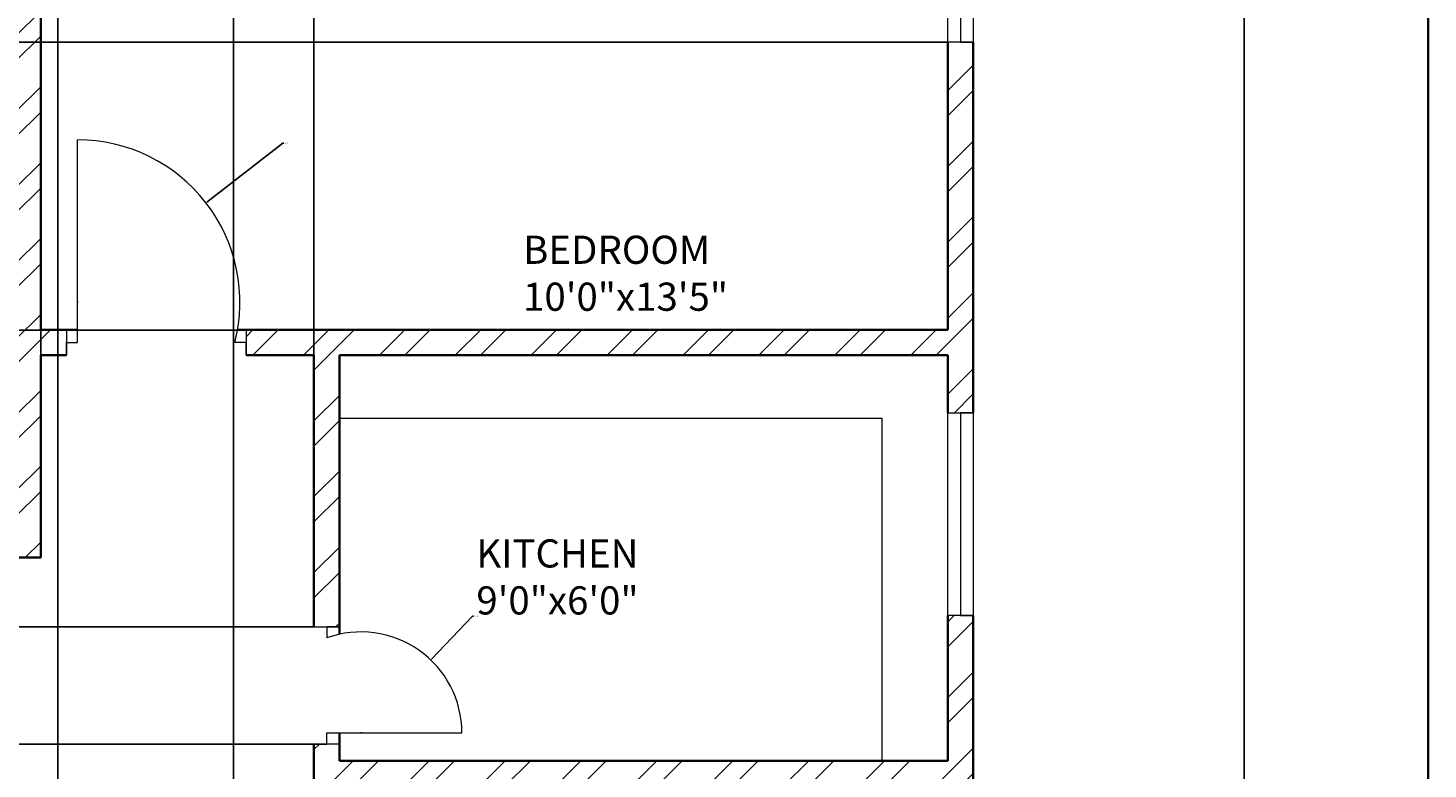
# Model space of a CAD drawing. Units: inches. Extents: x 2008 to 2657, y 1077 to 2165.
# Tile 15 of 16: x 2409 to 2657, y 1805 to 1937. Entities that reach past the tile are written whole.
import ezdxf

# ---------------------------------------------------------------- set-up
doc = ezdxf.new("R2010")
doc.units = ezdxf.units.IN
for name, color, linetype, lineweight in [('A-ANNO-DIMS', 2, 'Continuous', 18), ('A-ANNO-TTLB', 7, 'Continuous', 35), ('A-AREA-IDEN', 4, 'Continuous', 18), ('A-DOOR', 11, 'Continuous', 18), ('A-FLOR-CASE', 9, 'Continuous', 18), ('A-GLAZ', 191, 'Continuous', 18), ('A-WALL', 7, 'Continuous', 35)]:
    doc.layers.add(name, color=color, linetype=linetype, lineweight=lineweight)
doc.layers.add('A-WALL-PATT', color=30, linetype='Continuous', lineweight=13, true_color=0xf8991e)
doc.styles.get("Standard").update_dxf_attribs({"font": 'arial.ttf'})
doc.dimstyles.get("Standard").update_dxf_attribs({"dimtxt": 0.18, "dimasz": 0.18, "dimexe": 0.18, "dimexo": 0.0625, "dimgap": 0.09, "dimtad": 0, "dimtih": 1, "dimtoh": 1, "dimdec": 4, "dimzin": 0, "dimdsep": 46, "dimtxsty": 'Standard', "dimcen": 0.09, "dimadec": 0, "dimazin": 0, "dimtfac": 1, "dimtdec": 4, "dimtofl": 0, "dimtmove": 0, "dimatfit": 3, "dimfxl": 1, "dimtolj": 1, "dimtzin": 0, "dimarcsym": 0})

# ---------------------------------------------------------------- blocks, each defined once
blk = doc.blocks.new('WIN-60IN-B')
for p, q in [((0, 4.5), (0, 0)), ((0, 4.5), (60, 4.5)), ((60, 2.25), (60, 4.5)), ((60, 4.5), (60, 0)), ((0, 0), (0, 2.25)), ((0, 2.25), (60, 2.25)), ((60, 0), (0, 0))]:
    blk.add_line(p, q)
blk = doc.blocks.new('WIN-36IN-A')
for p, q in [((0, 36), (4.5, 36)), ((0, 0), (0, 36)), ((4.5, 36), (2.25, 36)), ((2.25, 36), (2.25, 0)), ((4.5, 36), (4.5, 0)), ((4.5, 0), (0, 0)), ((2.25, 0), (4.5, 0))]:
    blk.add_line(p, q)
blk = doc.blocks.new('*D32')
at = {"layer": 'A-ANNO-DIMS', "color": 0, "lineweight": -2, "transparency": 16777216}
for p, q in [((2576.82, 2094.67), (2624.99, 2094.67)), ((2624.81, 2094.49), (2624.81, 1641.86)), ((2624.81, 1188.85), (2624.81, 1641.49)), ((2576.82, 1188.67), (2624.99, 1188.67))]:
    blk.add_line(p, q, dxfattribs=at)
at = {"layer": 'A-ANNO-DIMS', "color": 0, "transparency": 16777216}
for points in [[(2624.78, 2094.49), (2624.84, 2094.49), (2624.81, 2094.67)], [(2624.78, 1188.85), (2624.84, 1188.85), (2624.81, 1188.67)]]:
    blk.add_solid(points, dxfattribs=at)
at = {"layer": 'Defpoints', "color": 0, "transparency": 16777216}
for p in [(2576.76, 2094.67), (2624.81, 2094.67), (2576.76, 1188.67)]:
    blk.add_point(p, dxfattribs=at)
at = {"layer": 'A-ANNO-DIMS', "color": 0, "transparency": 16777216, "insert": (2624.81, 1641.67), "char_height": 0.18, "attachment_point": 5}
blk.add_mtext('\\A1;906', dxfattribs=at)
blk = doc.blocks.new('*D56')
at = {"layer": 'A-ANNO-DIMS', "color": 0, "lineweight": -2, "transparency": 16777216}
for p, q in [((2411.26, 1842.83), (2411.26, 2142.9)), ((2411.44, 2142.72), (2435.18, 2142.72)), ((2459.58, 2142.72), (2435.84, 2142.72)), ((2459.76, 1830.56), (2459.76, 2142.9))]:
    blk.add_line(p, q, dxfattribs=at)
at = {"layer": 'A-ANNO-DIMS', "color": 0, "transparency": 16777216}
for points in [[(2411.44, 2142.75), (2411.44, 2142.69), (2411.26, 2142.72)], [(2459.58, 2142.75), (2459.58, 2142.69), (2459.76, 2142.72)]]:
    blk.add_solid(points, dxfattribs=at)
at = {"layer": 'Defpoints', "color": 0, "transparency": 16777216}
for p in [(2459.76, 2142.72), (2411.26, 1842.77), (2459.76, 1830.5)]:
    blk.add_point(p, dxfattribs=at)
at = {"layer": 'A-ANNO-DIMS', "color": 0, "transparency": 16777216, "insert": (2435.51, 2142.72), "char_height": 0.18, "attachment_point": 5}
blk.add_mtext('\\A1;48.5', dxfattribs=at)
blk = doc.blocks.new('*D57')
at = {"layer": 'A-ANNO-DIMS', "color": 0, "lineweight": -2, "transparency": 16777216}
for p, q in [((2414.28, 1754.24), (2414.28, 2142.9)), ((2414.46, 2142.72), (2429.47, 2142.72)), ((2445.27, 2142.72), (2430.26, 2142.72)), ((2445.45, 1751.99), (2445.45, 2142.9))]:
    blk.add_line(p, q, dxfattribs=at)
at = {"layer": 'A-ANNO-DIMS', "color": 0, "transparency": 16777216}
for points in [[(2414.46, 2142.75), (2414.46, 2142.69), (2414.28, 2142.72)], [(2445.27, 2142.75), (2445.27, 2142.69), (2445.45, 2142.72)]]:
    blk.add_solid(points, dxfattribs=at)
at = {"layer": 'Defpoints', "color": 0, "transparency": 16777216}
for p in [(2445.45, 2142.72), (2414.28, 1754.17), (2445.45, 1751.92)]:
    blk.add_point(p, dxfattribs=at)
at = {"layer": 'A-ANNO-DIMS', "color": 0, "transparency": 16777216, "insert": (2429.87, 2142.72), "char_height": 0.18, "attachment_point": 5}
blk.add_mtext('\\A1;31.17', dxfattribs=at)
blk = doc.blocks.new('*D58')
at = {"layer": 'A-ANNO-DIMS', "color": 0, "lineweight": -2, "transparency": 16777216}
for p, q in [((2459.7, 1830.5), (2028.03, 1830.5)), ((2028.21, 1830.32), (2028.21, 1820.26)), ((2028.21, 1809.84), (2028.21, 1819.9)), ((2459.7, 1809.66), (2028.03, 1809.66))]:
    blk.add_line(p, q, dxfattribs=at)
at = {"layer": 'A-ANNO-DIMS', "color": 0, "transparency": 16777216}
for points in [[(2028.18, 1830.32), (2028.24, 1830.32), (2028.21, 1830.5)], [(2028.18, 1809.84), (2028.24, 1809.84), (2028.21, 1809.66)]]:
    blk.add_solid(points, dxfattribs=at)
at = {"layer": 'Defpoints', "color": 0, "transparency": 16777216}
for p in [(2028.21, 1830.5), (2459.76, 1830.5), (2459.76, 1809.66)]:
    blk.add_point(p, dxfattribs=at)
at = {"layer": 'A-ANNO-DIMS', "color": 0, "transparency": 16777216, "insert": (2028.21, 1820.08), "char_height": 0.18, "attachment_point": 5}
blk.add_mtext('\\A1;20.835', dxfattribs=at)
blk = doc.blocks.new('*D67')
at = {"layer": 'A-ANNO-DIMS', "color": 0, "lineweight": -2, "transparency": 16777216}
for p, q in [((2572.2, 1934.29), (2028.03, 1934.29)), ((2028.21, 1934.11), (2028.21, 1908.91)), ((2028.21, 1883.35), (2028.21, 1908.55)), ((2572.2, 1883.17), (2028.03, 1883.17))]:
    blk.add_line(p, q, dxfattribs=at)
at = {"layer": 'A-ANNO-DIMS', "color": 0, "transparency": 16777216}
for points in [[(2028.18, 1934.11), (2028.24, 1934.11), (2028.21, 1934.29)], [(2028.18, 1883.35), (2028.24, 1883.35), (2028.21, 1883.17)]]:
    blk.add_solid(points, dxfattribs=at)
at = {"layer": 'Defpoints', "color": 0, "transparency": 16777216}
for p in [(2028.21, 1934.29), (2572.26, 1934.29), (2572.26, 1883.17)]:
    blk.add_point(p, dxfattribs=at)
at = {"layer": 'A-ANNO-DIMS', "color": 0, "transparency": 16777216, "insert": (2028.21, 1908.73), "char_height": 0.18, "attachment_point": 5}
blk.add_mtext('\\A1;51.11', dxfattribs=at)
blk = doc.blocks.new('*D72')
at = {"layer": 'A-ANNO-DIMS', "color": 0, "lineweight": -2, "transparency": 16777216}
for p, q in [((2454.25, 1916.34), (2440.73, 1905.87)), ((2454.43, 1916.34), (2454.25, 1916.34)), ((2417.73, 1888.13), (2417.91, 1888.13)), ((2417.82, 1888.04), (2417.82, 1888.22))]:
    blk.add_line(p, q, dxfattribs=at)
at = {"layer": 'A-ANNO-DIMS', "color": 0, "transparency": 16777216}
blk.add_solid([(2440.71, 1905.89), (2440.75, 1905.85), (2440.59, 1905.76)], dxfattribs=at)
at = {"layer": 'Defpoints', "color": 0, "transparency": 16777216}
for p in [(2440.59, 1905.76), (2417.82, 1888.13)]:
    blk.add_point(p, dxfattribs=at)
at = {"layer": 'A-ANNO-DIMS', "color": 0, "transparency": 16777216, "insert": (2454.84, 1916.34), "char_height": 0.18, "attachment_point": 5}
blk.add_mtext('\\A1;R28.8', dxfattribs=at)
blk = doc.blocks.new('*D88')
at = {"layer": 'A-ANNO-DIMS', "color": 0, "lineweight": -2, "transparency": 16777216}
for p, q in [((2487.89, 1832.39), (2480.59, 1824.74)), ((2488.07, 1832.39), (2487.89, 1832.39)), ((2468.02, 1811.66), (2468.2, 1811.66)), ((2468.11, 1811.57), (2468.11, 1811.75))]:
    blk.add_line(p, q, dxfattribs=at)
at = {"layer": 'A-ANNO-DIMS', "color": 0, "transparency": 16777216}
blk.add_solid([(2480.57, 1824.77), (2480.62, 1824.72), (2480.47, 1824.61)], dxfattribs=at)
at = {"layer": 'Defpoints', "color": 0, "transparency": 16777216}
for p in [(2480.47, 1824.61), (2468.11, 1811.66)]:
    blk.add_point(p, dxfattribs=at)
at = {"layer": 'A-ANNO-DIMS', "color": 0, "transparency": 16777216, "insert": (2488.62, 1832.39), "char_height": 0.18, "attachment_point": 5}
blk.add_mtext('\\A1;R17.905', dxfattribs=at)

msp = doc.modelspace()

# ---------------------------------------------------------------- hatches: boundary and pattern name
at = {"layer": 'A-WALL-PATT'}
h = msp.add_hatch(dxfattribs=at)
h.set_pattern_fill('ANSI32', color=256)
h.paths.add_polyline_path([(2109.2619, 2094.6743), (2104.7619, 2094.6743), (2104.7619, 2072.1743), (2104.7619, 2021.6151), (2109.2619, 2021.6151), (2109.2619, 2055.6743), (2126.1387, 2055.6743), (2126.1387, 2057.9243), (2126.1387, 2060.1743), (2109.2619, 2060.1743)])
h.paths.add_polyline_path([(2223.2494, 2057.9243), (2223.2494, 2060.1743), (2186.1387, 2060.1743), (2186.1387, 2055.6743), (2223.2494, 2055.6743)])
h.paths.add_polyline_path([(2250.7619, 2072.1743), (2250.7619, 2090.1743), (2250.7619, 2094.6743), (2246.2619, 2094.6743), (2246.2619, 2060.1743), (2242.7242, 2060.1743), (2242.7242, 2055.6743), (2246.2619, 2055.6743), (2246.2619, 1899.6743), (2242.7458, 1899.6743), (2242.7458, 1897.4243), (2242.7458, 1895.1743), (2246.2619, 1895.1743), (2246.2619, 1878.8745), (2248.5119, 1878.8745), (2250.7619, 1878.8745), (2250.7619, 1991.1743), (2250.7619, 2025.6743), (2257.6798, 2025.6743), (2257.6798, 2027.9243), (2257.6798, 2030.1743), (2250.7619, 2030.1743)])
h.paths.add_polyline_path([(2411.2619, 2031.6743), (2409.0119, 2031.6743), (2406.7619, 2031.6743), (2406.7619, 2030.1743), (2322.7619, 2030.1743), (2322.7619, 2053.3443), (2318.2619, 2053.3443), (2318.2619, 2030.1743), (2305.6798, 2030.1743), (2305.6798, 2025.6743), (2318.2619, 2025.6743), (2322.7619, 2025.6743), (2406.7619, 2025.6743), (2406.7619, 1995.6743), (2406.7619, 1847.2677), (2250.7619, 1847.2677), (2250.7619, 1850.9902), (2248.5119, 1850.9902), (2246.2619, 1850.9902), (2246.2619, 1847.1743), (2246.2619, 1842.7677), (2303.0015, 1842.7677), (2303.0015, 1667.2413), (2298.4208, 1667.2413), (2298.4208, 1662.7413), (2303.0015, 1662.7413), (2303.0015, 1649.8758), (2307.5015, 1649.8758), (2307.5015, 1842.7677), (2406.7619, 1842.7677), (2411.2619, 1842.7677), (2411.2619, 1878.6743), (2415.8196, 1878.6743), (2415.8196, 1880.9243), (2415.8196, 1883.1743), (2411.2619, 1883.1743)])
h.paths.add_polyline_path([(2411.2619, 2094.6743), (2406.7619, 2094.6743), (2318.2619, 2094.6743), (2318.2619, 2077.3443), (2322.7619, 2077.3443), (2322.7619, 2090.1743), (2406.7619, 2090.1743), (2406.7619, 2072.1743), (2406.7619, 2067.6743), (2406.7619, 2052.7524), (2411.2619, 2052.7524), (2411.2619, 2055.6743), (2414.9888, 2055.6743), (2414.9888, 2057.9243), (2414.9888, 2060.1743), (2411.2619, 2060.1743), (2411.2619, 2072.1743)])
h.paths.add_polyline_path([(2576.7619, 2072.1743), (2576.7619, 2094.6743), (2572.2619, 2094.6743), (2572.2619, 2060.1743), (2525.8113, 2060.1743), (2525.8113, 2055.6743), (2572.2619, 2055.6743), (2572.2619, 1994.289), (2576.7619, 1994.289)])
h.paths.add_polyline_path([(2465.8113, 2060.1743), (2436.2802, 2060.1743), (2436.2802, 2055.6743), (2465.8113, 2055.6743), (2465.8113, 2057.9243)])
h.paths.add_polyline_path([(2576.7619, 1934.289), (2574.5119, 1934.289), (2572.2619, 1934.289), (2572.2619, 1883.1743), (2447.7027, 1883.1743), (2447.7027, 1878.6743), (2459.7619, 1878.6743), (2459.7619, 1830.4982), (2464.2619, 1830.4982), (2464.2619, 1878.6743), (2572.2619, 1878.6743), (2572.2619, 1868.4883), (2576.7619, 1868.4883)])
h.paths.add_polyline_path([(2576.7619, 1832.4883), (2572.2619, 1832.4883), (2572.2619, 1806.6743), (2464.2619, 1806.6743), (2464.2619, 1809.6629), (2459.7619, 1809.6629), (2459.7619, 1802.1743), (2483.7619, 1802.1743), (2483.7619, 1778.1743), (2488.2619, 1778.1743), (2488.2619, 1802.1743), (2572.2619, 1802.1743), (2572.2619, 1793.6101), (2576.7619, 1793.6101)])
h.paths.add_polyline_path([(2576.7619, 1769.6101), (2572.2619, 1769.6101), (2572.2619, 1754.1743), (2488.2619, 1754.1743), (2488.2619, 1757.2675), (2486.0119, 1757.2675), (2483.7619, 1757.2675), (2483.7619, 1754.1743), (2447.4528, 1754.1743), (2447.4528, 1749.6743), (2483.7619, 1749.6743), (2572.2619, 1749.6743), (2572.2619, 1715.1837), (2576.7619, 1715.1837)])
h.paths.add_polyline_path([(2576.7619, 1655.1837), (2572.2619, 1655.1837), (2572.2619, 1617.6743), (2411.2619, 1617.6743), (2411.2619, 1749.6743), (2414.2827, 1749.6743), (2414.2827, 1754.1743), (2406.7619, 1754.1743), (2406.7619, 1749.6743), (2406.7619, 1617.6743), (2307.5015, 1617.6743), (2307.5015, 1621.0007), (2305.2515, 1621.0007), (2303.0015, 1621.0007), (2303.0015, 1609.6944), (2307.5015, 1609.6944), (2307.5015, 1613.1743), (2406.7619, 1613.1743), (2406.7619, 1476.6743), (2415.532, 1476.6743), (2415.532, 1478.9243), (2415.532, 1481.1743), (2411.2619, 1481.1743), (2411.2619, 1613.1743), (2572.2619, 1613.1743), (2572.2619, 1584.6086), (2576.7619, 1584.6086)])
h.paths.add_polyline_path([(2576.7619, 1524.6086), (2572.2619, 1524.6086), (2572.2619, 1481.1743), (2483.7619, 1481.1743), (2447.5119, 1481.1743), (2447.5119, 1476.6743), (2483.7619, 1476.6743), (2483.7619, 1473.5051), (2488.2619, 1473.5051), (2488.2619, 1476.6743), (2572.2619, 1476.6743), (2572.2619, 1469.5488), (2576.7619, 1469.5488)])
h.paths.add_polyline_path([(2576.7619, 1445.5488), (2572.2619, 1445.5488), (2572.2619, 1428.6743), (2488.2619, 1428.6743), (2488.2619, 1455.6743), (2486.0119, 1455.6743), (2483.7619, 1455.6743), (2483.7619, 1428.6743), (2459.7619, 1428.6743), (2459.7619, 1422.1519), (2464.2619, 1422.1519), (2464.2619, 1424.1743), (2572.2619, 1424.1743), (2572.2619, 1407.5685), (2576.7619, 1407.5685)])
h.paths.add_polyline_path([(2576.7619, 1371.5685), (2572.2619, 1371.5685), (2572.2619, 1352.1743), (2464.2619, 1352.1743), (2464.2619, 1403.1384), (2462.0119, 1403.1384), (2459.7619, 1403.1384), (2459.7619, 1352.1743), (2446.3194, 1352.1743), (2446.3194, 1347.6743), (2572.2619, 1347.6743), (2572.2619, 1321.0291), (2576.7619, 1321.0291)])
h.paths.add_polyline_path([(2462.703, 1227.6743), (2436.0298, 1227.6743), (2436.0298, 1225.4243), (2436.0298, 1223.1743), (2462.703, 1223.1743), (2462.703, 1225.4243)])
h.paths.add_polyline_path([(2576.7619, 1261.0291), (2574.5119, 1261.0291), (2572.2619, 1261.0291), (2572.2619, 1227.6743), (2522.703, 1227.6743), (2522.703, 1223.1743), (2572.2619, 1223.1743), (2572.2619, 1188.6743), (2576.7619, 1188.6743), (2576.7619, 1193.1743), (2576.7619, 1223.1743)])
h.paths.add_polyline_path([(2414.2823, 1227.6743), (2411.2619, 1227.6743), (2411.2619, 1267.1779), (2409.0119, 1267.1779), (2406.7619, 1267.1779), (2406.7619, 1227.6743), (2322.7619, 1227.6743), (2322.7619, 1244.3623), (2318.2619, 1244.3623), (2318.2619, 1223.1743), (2406.7619, 1223.1743), (2406.7619, 1193.1743), (2406.7619, 1188.6743), (2411.2619, 1188.6743), (2411.2619, 1193.1743), (2411.2619, 1223.1743), (2414.2823, 1223.1743)])
h.paths.add_polyline_path([(2411.2619, 1347.6743), (2414.702, 1347.6743), (2414.702, 1349.9243), (2414.702, 1352.1743), (2411.2619, 1352.1743), (2411.2619, 1416.7413), (2307.5015, 1416.7413), (2307.5015, 1579.8489), (2305.2515, 1579.8489), (2303.0015, 1579.8489), (2303.0015, 1566.7413), (2299.2719, 1566.7413), (2299.2719, 1562.2413), (2303.0015, 1562.2413), (2303.0015, 1416.7413), (2246.2619, 1416.7413), (2246.2619, 1409.8616), (2250.7619, 1409.8616), (2250.7619, 1412.2413), (2406.7619, 1412.2413), (2406.7619, 1292.1743), (2304.9703, 1292.1743), (2304.9703, 1287.6743), (2318.2619, 1287.6743), (2318.2619, 1268.3623), (2322.7619, 1268.3623), (2322.7619, 1287.6743), (2406.7619, 1287.6743), (2406.7619, 1285.4748), (2411.2619, 1285.4748)])
h.paths.add_polyline_path([(2109.2619, 1262.7482), (2104.7619, 1262.7482), (2104.7619, 1223.1743), (2104.7619, 1193.1743), (2104.7619, 1188.6743), (2109.2619, 1188.6743), (2109.2619, 1223.1743), (2126.7928, 1223.1743), (2126.7928, 1225.4243), (2126.7928, 1227.6743), (2109.2619, 1227.6743)])
h.paths.add_polyline_path([(2222.3268, 1227.6743), (2186.7928, 1227.6743), (2186.7928, 1223.1743), (2222.3268, 1223.1743)])
h.paths.add_polyline_path([(2250.7619, 1287.6743), (2256.9703, 1287.6743), (2256.9703, 1289.9243), (2256.9703, 1292.1743), (2250.7619, 1292.1743), (2250.7619, 1382.2078), (2248.5119, 1382.2078), (2246.2619, 1382.2078), (2246.2619, 1347.6743), (2246.2619, 1227.6743), (2242.6068, 1227.6743), (2242.6068, 1223.1743), (2246.2619, 1223.1743), (2246.2619, 1188.6743), (2250.7619, 1188.6743), (2250.7619, 1193.1743), (2250.7619, 1227.6743)])
h.paths.add_polyline_path([(2133.2619, 1349.9243), (2133.2619, 1352.1743), (2109.2619, 1352.1743), (2109.2619, 1375.2826), (2104.7619, 1375.2826), (2104.7619, 1322.7482), (2109.2619, 1322.7482), (2109.2619, 1347.6743), (2133.2619, 1347.6743)])
h.paths.add_polyline_path([(2210.2105, 1352.1743), (2161.7619, 1352.1743), (2161.7619, 1412.2413), (2185.7619, 1412.2413), (2185.7619, 1420.1851), (2183.5119, 1420.1851), (2181.2619, 1420.1851), (2181.2619, 1416.7413), (2109.2619, 1416.7413), (2109.2619, 1452.4006), (2104.7619, 1452.4006), (2104.7619, 1399.2826), (2109.2619, 1399.2826), (2109.2619, 1412.2413), (2157.2619, 1412.2413), (2157.2619, 1352.1743), (2154.3383, 1352.1743), (2154.3383, 1347.6743), (2210.2105, 1347.6743)])
h.paths.add_polyline_path([(2185.7619, 1514.2413), (2161.7619, 1514.2413), (2161.7619, 1518.1307), (2159.5119, 1518.1307), (2157.2619, 1518.1307), (2157.2619, 1514.2413), (2109.2619, 1514.2413), (2109.2619, 1528.997), (2107.0119, 1528.997), (2104.7619, 1528.997), (2104.7619, 1488.4006), (2109.2619, 1488.4006), (2109.2619, 1509.7413), (2181.2619, 1509.7413), (2181.2619, 1441.2042), (2185.7619, 1441.2042)])
h.paths.add_polyline_path([(2270.4025, 1566.7413), (2109.2619, 1566.7413), (2080.7619, 1566.7413), (2080.7619, 1586.5643), (2076.2619, 1586.5643), (2076.2619, 1562.2413), (2080.7619, 1562.2413), (2104.7619, 1562.2413), (2104.7619, 1552.997), (2109.2619, 1552.997), (2109.2619, 1562.2413), (2157.2619, 1562.2413), (2157.2619, 1538.2413), (2161.7619, 1538.2413), (2161.7619, 1562.2413), (2205.2619, 1562.2413), (2270.4025, 1562.2413)])
h.paths.add_polyline_path([(2131.6813, 1897.4243), (2131.6813, 1899.6743), (2109.2619, 1899.6743), (2109.2619, 1961.6151), (2104.7619, 1961.6151), (2104.7619, 1886.8042), (2109.2619, 1886.8042), (2109.2619, 1895.1743), (2131.6813, 1895.1743)])
h.paths.add_polyline_path([(2185.7619, 1847.1743), (2161.7619, 1847.1743), (2161.7619, 1895.1743), (2185.7619, 1895.1743), (2211.543, 1895.1743), (2211.543, 1897.4243), (2211.543, 1899.6743), (2154.0916, 1899.6743), (2154.0916, 1897.4243), (2154.0916, 1895.1743), (2157.2619, 1895.1743), (2157.2619, 1847.1743), (2109.2619, 1847.1743), (2109.2619, 1862.8042), (2104.7619, 1862.8042), (2104.7619, 1821.243), (2109.2619, 1821.243), (2109.2619, 1842.6743), (2181.2619, 1842.6743), (2181.2619, 1840.6763), (2185.7619, 1840.6763)])
h.paths.add_polyline_path([(2109.2619, 1785.243), (2104.7619, 1785.243), (2104.7619, 1715.4691), (2109.2619, 1715.4691), (2109.2619, 1730.8423), (2157.2619, 1730.8423), (2157.2619, 1727.6404), (2161.7619, 1727.6404), (2161.7619, 1730.8423), (2185.7619, 1730.8423), (2185.7619, 1822.1438), (2183.5119, 1822.1438), (2181.2619, 1822.1438), (2181.2619, 1735.3423), (2109.2619, 1735.3423)])
h.paths.add_polyline_path([(2109.2619, 1691.4691), (2104.7619, 1691.4691), (2104.7619, 1667.2413), (2076.2619, 1667.2413), (2076.2619, 1646.5643), (2080.7619, 1646.5643), (2080.7619, 1662.7413), (2109.2619, 1662.7413), (2271.4941, 1662.7413), (2271.4941, 1664.9913), (2271.4941, 1667.2413), (2181.2619, 1667.2413), (2161.7619, 1667.2413), (2161.7619, 1708.3752), (2159.5119, 1708.3752), (2157.2619, 1708.3752), (2157.2619, 1667.2413), (2109.2619, 1667.2413)])
h.paths.add_polyline_path([(2233.1467, 1747.4973), (2270.0737, 1747.4973), (2270.0737, 1766.1547), (2233.1467, 1766.1547)], flags=9)

# ---------------------------------------------------------------- linework, layer by layer
at = {"layer": 'A-ANNO-TTLB'}
msp.add_lwpolyline([(2008.4537, 2164.5615), (2657.4477, 2164.5615), (2657.4477, 1076.8888), (2008.4537, 1076.8888)], close=True, dxfattribs=at)
at = {"layer": 'A-DOOR'}
for p, q in [((2417.8196, 1880.9243), (2417.8196, 1916.9243)), ((2415.8196, 1883.1743), (2415.8196, 1878.6743)), ((2447.7027, 1883.1743), (2447.7027, 1878.6743)), ((2415.8196, 1878.6743), (2415.8196, 1880.9243)), ((2415.8196, 1880.9243), (2417.8196, 1880.9243)), ((2447.7027, 1880.9243), (2445.7027, 1880.9243)), ((2447.7027, 1878.6743), (2447.7027, 1880.9243)), ((2459.7619, 1830.4982), (2464.2619, 1830.4982)), ((2464.2619, 1830.4982), (2462.0119, 1830.4982)), ((2462.0119, 1830.4982), (2462.0119, 1828.4982)), ((2462.0119, 1809.6629), (2462.0119, 1811.6629)), ((2462.0119, 1811.6629), (2486.0119, 1811.6629)), ((2464.2619, 1809.6629), (2459.7619, 1809.6629)), ((2459.7619, 1809.6629), (2462.0119, 1809.6629))]:
    msp.add_line(p, q, dxfattribs=at)
for centre, radius, start, end in [((2417.8196, 1888.1262), 28.7981, 345.517596, 90), ((2468.1072, 1811.6629), 17.9047, 360, 109.902868)]:
    msp.add_arc(centre, radius, start, end, dxfattribs=at)
at = {"layer": 'A-FLOR-CASE'}
for p, q in [((2464.2619, 1867.5128), (2560.5188, 1867.5128)), ((2560.5188, 1867.5128), (2560.5188, 1806.6743))]:
    msp.add_line(p, q, dxfattribs=at)
at = {"layer": 'A-WALL'}
for p, q in [((2411.2619, 2031.6743), (2411.2619, 1883.1743)), ((2572.2619, 1934.289), (2572.2619, 1883.1743)), ((2576.7619, 1934.289), (2576.7619, 1868.4883)), ((2572.2619, 1895.1743), (2572.2619, 1883.1743)), ((2411.2619, 1883.1743), (2417.8196, 1883.1743)), ((2446.1888, 1883.1743), (2572.2619, 1883.1743)), ((2411.2619, 1878.6743), (2415.8196, 1878.6743)), ((2411.2619, 1878.6743), (2411.2619, 1842.7677)), ((2447.7027, 1878.6743), (2459.7619, 1878.6743)), ((2459.7619, 1878.6743), (2459.7619, 1830.4982)), ((2464.2619, 1878.6743), (2464.2619, 1829.1499)), ((2464.2619, 1878.6743), (2572.2619, 1878.6743)), ((2572.2619, 1878.6743), (2572.2619, 1868.4883)), ((2406.7619, 1842.7677), (2411.2619, 1842.7677)), ((2572.2619, 1832.4883), (2572.2619, 1806.6743)), ((2576.7619, 1832.4883), (2576.7619, 1793.6101)), ((2464.2619, 1811.6629), (2464.2619, 1806.6743)), ((2459.7619, 1809.6629), (2459.7619, 1802.1743)), ((2464.2619, 1806.6743), (2572.2619, 1806.6743))]:
    msp.add_line(p, q, dxfattribs=at)

# ---------------------------------------------------------------- block references
at = {"layer": 'A-GLAZ', "rotation": 270.0000000000001}
msp.add_blockref('WIN-60IN-B', (2572.2616, 1994.2888), dxfattribs=at)
at = {"layer": 'A-GLAZ'}
msp.add_blockref('WIN-36IN-A', (2572.262, 1832.488), dxfattribs=at)

# ---------------------------------------------------------------- texts
at = {"layer": 'A-AREA-IDEN', "char_height": 5, "attachment_point": 1}
for s, width, insert in [('BEDROOM\\P10\'0"x13\'5"', 135.75227, (2496.8689, 1899.9149)), ('KITCHEN\\P9\'0"x6\'0"', 165.62191, (2488.5766, 1846.0034))]:
    msp.add_mtext_dynamic_manual_height_columns(s, width=width, gutter_width=12.5, heights=[0], dxfattribs=dict(at, insert=insert))

# ---------------------------------------------------------------- dimensions: what is measured, and where the dimension line sits
at = {"layer": 'A-ANNO-DIMS'}
for base, p1, p2, override, picture, middle in [((2459.7619, 2142.7243), (2411.2619, 1842.7677), (2459.7619, 1830.4982), {"dimdec": 1, "dimlfac": 1, "dimrnd": 0, "dimzin": 0, "dimdsep": 46, "dimlunit": 2}, '*D56', (2435.5119, 2142.7243)), ((2445.4528, 2142.7243), (2414.2827, 1754.1743), (2445.4528, 1751.9243), {"dimdec": 2, "dimlfac": 1, "dimrnd": 0, "dimzin": 0, "dimdsep": 46, "dimlunit": 2}, '*D57', (2429.8677, 2142.7243))]:
    dim = msp.add_linear_dim(base=base, p1=p1, p2=p2, dimstyle='Standard', override=override, dxfattribs=at)
    dim.commit()
    dim.dimension.update_dxf_attribs({"geometry": picture, "text_midpoint": middle})
for base, p1, p2, override, picture, middle in [((2624.8119, 2094.6743), (2576.7619, 1188.6743), (2576.7619, 2094.6743), {"dimdec": 0, "dimlfac": 1, "dimrnd": 0, "dimzin": 0, "dimdsep": 46, "dimlunit": 2}, '*D32', (2624.8119, 1641.6743)), ((2028.2119, 1934.289), (2572.2619, 1883.1743), (2572.2619, 1934.289), {"dimdec": 2, "dimlfac": 1, "dimrnd": 0, "dimzin": 0, "dimdsep": 46, "dimlunit": 2}, '*D67', (2028.2119, 1908.7317)), ((2028.2119, 1830.4982), (2459.7619, 1809.6629), (2459.7619, 1830.4982), {"dimdec": 3, "dimlfac": 1, "dimrnd": 0, "dimzin": 0, "dimdsep": 46, "dimlunit": 2}, '*D58', (2028.2119, 1820.0806))]:
    dim = msp.add_linear_dim(base=base, p1=p1, p2=p2, angle=90, dimstyle='Standard', override=override, dxfattribs=at)
    dim.commit()
    dim.dimension.update_dxf_attribs({"geometry": picture, "text_midpoint": middle})
for center, mpoint, override, picture, middle in [((2417.8196, 1888.1262), (2440.5874, 1905.7603), {"dimdec": 1, "dimlfac": 1, "dimrnd": 0, "dimzin": 0, "dimdsep": 46, "dimlunit": 2}, '*D72', (2454.8381, 1916.3407)), ((2468.1072, 1811.6629), (2480.47, 1824.6143), {"dimdec": 3, "dimlfac": 1, "dimrnd": 0, "dimzin": 0, "dimdsep": 46, "dimlunit": 2}, '*D88', (2488.6182, 1832.3852))]:
    dim = msp.add_radius_dim(center=center, mpoint=mpoint, dimstyle='Standard', override=override, dxfattribs=at)
    dim.commit()
    dim.dimension.update_dxf_attribs({"geometry": picture, "text_midpoint": middle, "dimtype": 164})

doc.saveas('drawing.dxf')
